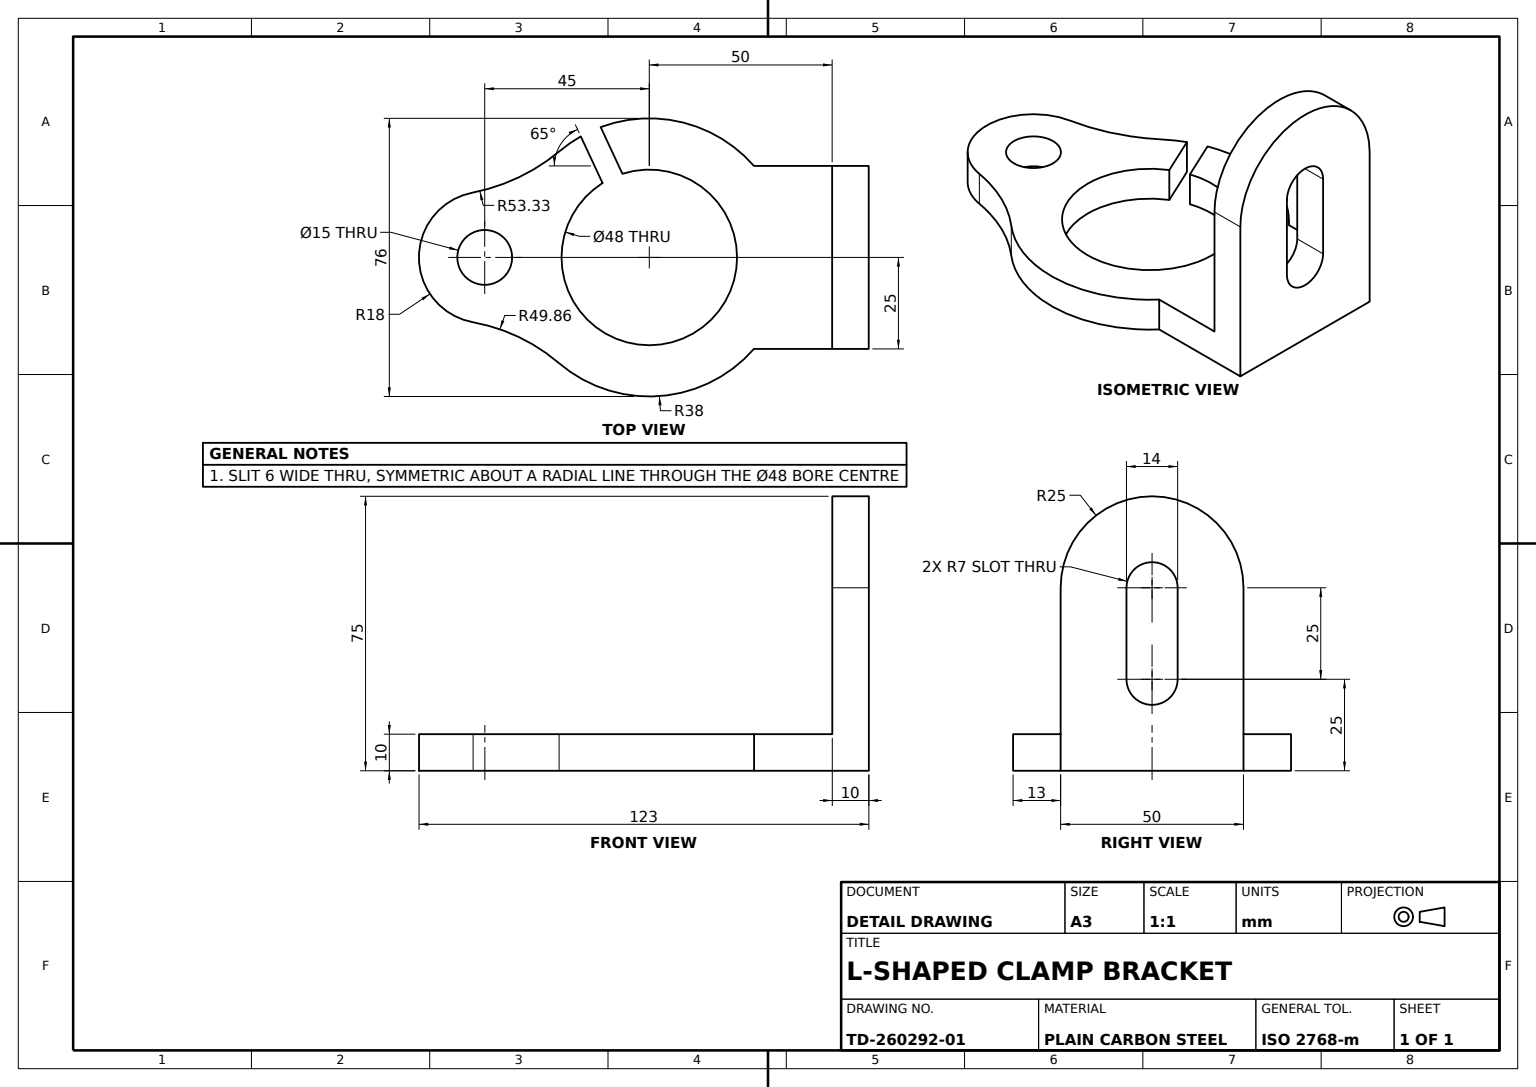
from build123d import *

# Parameters (mm, degrees)
CLAMP_BASE_PROFILE_SKETCH_R = 7.5
CLAMP_BASE_PLATE_DEPTH      = 5
SLOTTED_UPRIGHT_TAB_DEPTH   = 10


with BuildPart() as part:
    # Clamp Base Profile Sketch → Clamp Base Plate (new, symmetric)
    with BuildSketch(Plane(origin=(0, 0, 0), x_dir=(1, 0, 0), z_dir=(0, 1, 0))):
        with BuildLine():
            Line((-25, -33.131068574), (-25, -11.749244617))
            Line((-25, -11.749244617), (25, -11.749244617))
            Line((25, -11.749244617), (25, -33.131068574))
            ThreePointArc((25, -33.131068574), (37.899800142, -58.991501114), (28.879478838, -86.446930784))
            ThreePointArc((28.879478838, -86.446930784), (21.733959657, -97.461955057), (17.711280988, -109.960245356))
            ThreePointArc((17.711280988, -109.960245356), (0.118395162, -124.74885524), (-17.667508621, -110.192954697))
            ThreePointArc((-17.667508621, -110.192954697), (-21.873782153, -97.444622756), (-29.130311117, -86.150576019))
            ThreePointArc((-29.130311117, -86.150576019), (-31.226426819, -83.403580628), (-33.064347445, -80.477536799))
            Line((-33.064347445, -80.477536799), (-20.312930357, -74.531453358))
            ThreePointArc((-20.312930357, -74.531453358), (21.751386889, -51.606406335), (-22.848639927, -69.093606636))
            Line((-22.848639927, -69.093606636), (-35.600057015, -75.039690077))
            ThreePointArc((-35.600057015, -75.039690077), (-36.839854324, -52.431244113), (-25, -33.131068574))
        make_face()
        with Locations(Location((0, -106.749244617, 0), (0, 0, 270))):
            Circle(CLAMP_BASE_PROFILE_SKETCH_R, mode=Mode.SUBTRACT)
    extrude(amount=CLAMP_BASE_PLATE_DEPTH, both=True)

    # Slotted Tab Profile Sketch → Slotted Upright Tab (add)
    with BuildSketch(Plane(origin=(0, 0, 11.749244617), x_dir=(-1, 0, 0), z_dir=(0, 0, -1))):
        with BuildLine():
            Line((-25, -5), (-25, 45))
            ThreePointArc((-25, 45), (0, 70), (25, 45))
            Line((25, 45), (25, -5))
            Line((25, -5), (-25, -5))
        make_face()
        with BuildLine():
            Line((7, 45), (7, 20))
            ThreePointArc((7, 20), (0, 13), (-7, 20))
            Line((-7, 20), (-7, 45))
            ThreePointArc((-7, 45), (0, 52), (7, 45))
        make_face(mode=Mode.SUBTRACT)
    extrude(amount=SLOTTED_UPRIGHT_TAB_DEPTH)


solid = part.part
